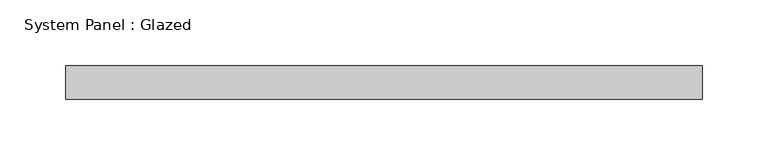
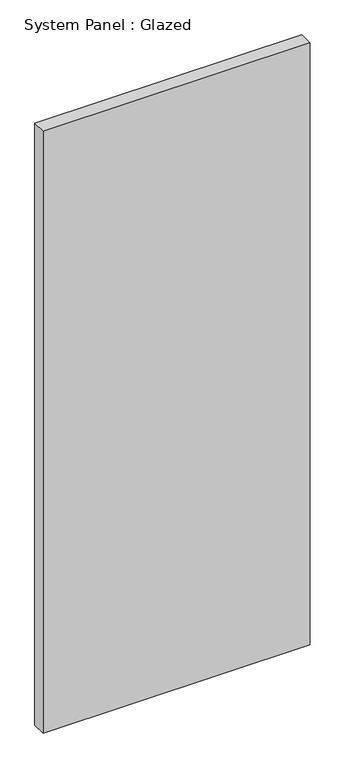
"""IFC4 building model written with IfcOpenShell, lengths in millimetres: plate geometry, System Panel : Glazed."""

from ifc_helpers import new_model, si_unit, origin, origin_with_axes, place, context, project, spatial, polyline, outline, extrude, source, transform, mapped, element, save


def system_panel_glazed_030ff9b4(model_context):
    return source(origin(), model_context, "Body", "SweptSolid", [
        extrude(outline(polyline([(241.3, 19.05), (-241.3, 19.05), (-241.3, 44.45), (241.3, 44.45), (241.3, 19.05)])), origin_with_axes(), (0.0, 0.0, 1.0), 1149.35),
    ])


if __name__ == "__main__":
    model = new_model("IFC4")
    model_context = context("Model", 3, world=origin())
    ifc_project = project(units=[si_unit("LENGTHUNIT", "METRE", prefix="MILLI")], contexts=[model_context])
    site = spatial("IfcSite", under=ifc_project)
    building = spatial("IfcBuilding", under=site)
    placement = place(None, origin())
    system_panel_glazed_shape = system_panel_glazed_030ff9b4(model_context)
    element("IfcPlate", 1, ObjectType="System Panel : Glazed", at=placement, inside=building, context=model_context, shape_type="MappedRepresentation", body=[
        mapped(system_panel_glazed_shape, transform((0.0, 0.0, 0.0), x_axis=(1.0, 0.0, 0.0), y_axis=(0.0, 1.0, 0.0), z_axis=(0.0, 0.0, 1.0))),
    ])
    save(model, "model.ifc")

# Revit data of these elements
# Type "System Panel : Glazed"
#   Construction Type Id = "GSP4R"
#   Analytic Construction = "1/8 in Pilkington single glazing"
#   Visual Light Transmittance = 0.9
#   Solar Heat Gain Coefficient = 0.86
#   Heat Transfer Coefficient (U) = 1.18115 BTU/(h·ft²·°F)
#   Define Thermal Properties by = 1
# Element 1 (IfcPlate, "System Panel : Glazed")
#   Materials on its faces: "Glass"
# Materials
#   "Glass": class "Glass", colour RGB 0 128 192, transparency 0.75, Description = "Soda Lime Glass", Cost = 0
